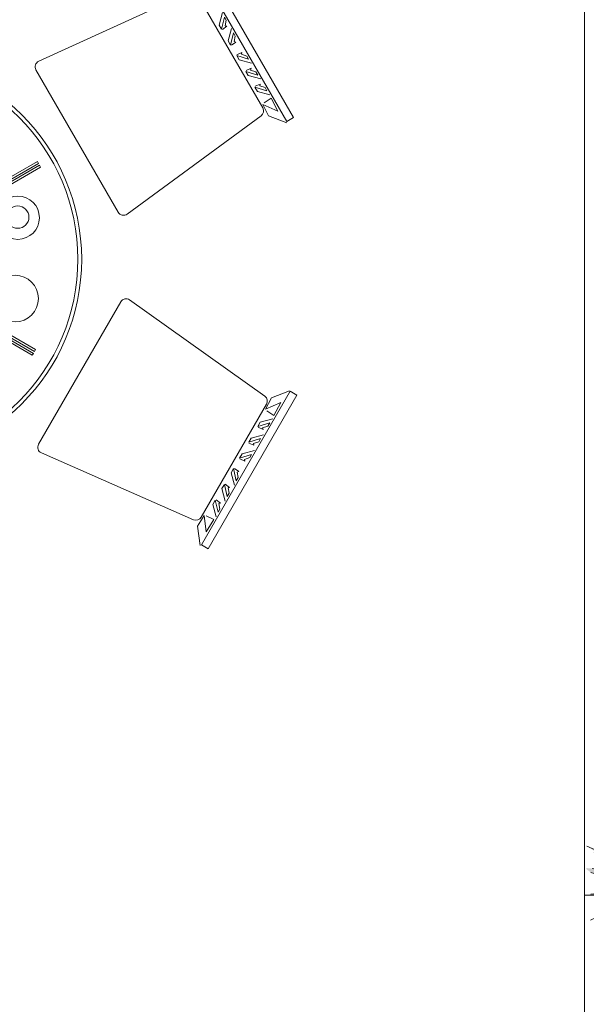
# Model space of a CAD drawing. Units: inches. Extents: x 1239 to 2276906, y 2273 to 321338.
# Tile 4 of 23: x 1482 to 1541, y 2408 to 2510. Entities that reach past the tile are written whole.
import ezdxf

# ---------------------------------------------------------------- set-up
doc = ezdxf.new("R2010")
doc.units = ezdxf.units.IN
for name, color, linetype, lineweight in [('A-ANNO-DIMS', 2, 'Continuous', 18), ('A-FURN', 8, 'Continuous', 13), ('L-PLNT', 94, 'Continuous', 13)]:
    doc.layers.add(name, color=color, linetype=linetype, lineweight=lineweight)
doc.styles.get("Standard").update_dxf_attribs({"font": 'arial.ttf'})
doc.dimstyles.new('ISO-25', dxfattribs={"dimtxt": 4.5, "dimasz": 4, "dimexe": 1.25, "dimexo": 0.625, "dimtad": 1, "dimdec": 1, "dimlunit": 3, "dimtxsty": 'Standard', "dimcen": 2.5, "dimadec": 0, "dimazin": 0, "dimtfac": 1, "dimtdec": 1, "dimtmove": 0, "dimatfit": 3, "dimfxl": 1, "dimarcsym": 0})

# ---------------------------------------------------------------- blocks, each defined once
blk = doc.blocks.new('A$C545C060E')
h = blk.add_hatch(color=256)
h.set_gradient(color1=(31, 127, 0), color2=(45, 179, 0), one_color=1, tint=0.35, name='INVSPHERICAL')
h.paths.add_polyline_path([(0.529, 2.393), (0.645, 2.304), (1.889, 1.967), (0.489, 1.77), (1.843, 1.787), (1.618, 1.643), (0.635, 1.178), (1.063, 1.326), (1.966, 1.643), (1.461, 1.231), (1.869, 1.417), (2.379, 1.664), (2.177, 1.5), (1.446, 1.03), (1.981, 1.358), (1.481, 0.744), (2.376, 1.553), (1.986, 0.848), (2.48, 1.336), (1.85, 0.496), (2.266, 0.842), (2.223, 0.533), (2.243, 0.142), (2.487, 1.093), (2.615, 0.257), (2.655, 1.214), (3.074, 0.284), (3.303, 0), (2.908, 1.003), (2.846, 1.271), (2.929, 1.199), (3.853, 0.038), (3.428, 0.832), (3.973, 0.376), (4.009, 0.393), (3.432, 1.008), (3.923, 0.676), (4.175, 0.507), (4.274, 0.474), (4.155, 0.583), (4.009, 0.757), (3.765, 0.932), (3.662, 1.051), (4.067, 0.828), (4.243, 0.779), (4.238, 0.801), (3.802, 1.133), (4.534, 0.795), (4.591, 0.795), (4.42, 0.899), (4.103, 1.12), (3.786, 1.34), (3.464, 1.533), (3.968, 1.441), (4.415, 1.362), (4.571, 1.335), (4.695, 1.33), (3.997, 1.572), (3.423, 1.771), (4.695, 1.782), (3.833, 1.912), (4.591, 2.011), (3.836, 2.079), (4.706, 2.305), (3.951, 2.263), (4.55, 2.506), (4.555, 2.528), (4.493, 2.517), (3.734, 2.332), (4.197, 2.577), (4.56, 2.833), (3.786, 2.523), (4.363, 2.959), (4.394, 2.997), (4.363, 2.997), (3.558, 2.528), (3.549, 2.536), (4.087, 3.155), (4.254, 3.422), (4.191, 3.389), (3.209, 2.381), (4.046, 3.912), (3.999, 3.874), (3.09, 2.626), (3.547, 3.58), (3.666, 3.934), (3.35, 3.438), (3.017, 2.752), (3.225, 3.411), (3.345, 4.064), (3.243, 3.868), (3.184, 3.754), (2.919, 3.073), (2.986, 3.83), (2.991, 4.097), (2.96, 4.075), (2.742, 2.981), (2.732, 2.92), (2.659, 4.026), (2.633, 4.092), (2.612, 4.005), (2.56, 2.719), (2.3, 4.135), (2.382, 2.743), (2.025, 4.026), (2.02, 3.934), (1.968, 3.917), (2.046, 3.874), (2.185, 2.776), (1.976, 3.197), (1.829, 3.524), (1.673, 3.773), (1.577, 3.963), (1.613, 3.821), (1.751, 3.44), (1.89, 3.059), (2.192, 2.446), (1.345, 3.551), (1.215, 3.683), (1.481, 3.234), (2.006, 2.515), (1.567, 2.769), (0.983, 3.176), (0.731, 3.334), (1.255, 2.901), (1.969, 2.294), (0.912, 2.769), (0.549, 2.927), (1.687, 2.199), (0.675, 2.399), (0.554, 2.409)])
h = blk.add_hatch(color=256)
h.set_gradient(color1=(31, 127, 0), color2=(55, 219, 0), one_color=1, tint=0.43, name='SPHERICAL')
h.paths.add_polyline_path([(3.023, 2.188), (3.114, 2.362), (3.471, 3.049), (3.33, 2.866), (2.618, 1.891), (2.679, 1.855), (2.94, 2.013)])
h = blk.add_hatch(color=256)
h.set_gradient(color1=(31, 127, 0), color2=(45, 179, 0), one_color=1, tint=0.35, name='INVSPHERICAL')
h.paths.add_polyline_path([(0.025, 1.517), (0.098, 1.461), (0.877, 1.25), (0, 1.126), (0.848, 1.137), (0.707, 1.047), (0.092, 0.756), (0.36, 0.848), (0.925, 1.047), (0.609, 0.789), (0.865, 0.905), (1.184, 1.06), (1.058, 0.958), (0.6, 0.663), (0.935, 0.868), (0.622, 0.484), (1.182, 0.99), (0.938, 0.549), (1.247, 0.855), (0.853, 0.328), (1.113, 0.545), (1.086, 0.352), (1.099, 0.106), (1.252, 0.703), (1.332, 0.179), (1.357, 0.779), (1.62, 0.195), (1.763, 0.018), (1.515, 0.646), (1.477, 0.814), (1.529, 0.769), (2.108, 0.042), (1.841, 0.539), (2.183, 0.253), (2.206, 0.264), (1.844, 0.649), (2.152, 0.441), (2.31, 0.335), (2.371, 0.315), (2.297, 0.383), (2.206, 0.492), (2.053, 0.602), (1.988, 0.676), (2.242, 0.537), (2.352, 0.506), (2.349, 0.52), (2.076, 0.728), (2.534, 0.516), (2.57, 0.516), (2.463, 0.581), (2.264, 0.719), (2.066, 0.857), (1.864, 0.978), (2.18, 0.921), (2.46, 0.871), (2.557, 0.854), (2.636, 0.851), (2.198, 1.003), (1.839, 1.127), (2.636, 1.134), (2.095, 1.216), (2.57, 1.277), (2.097, 1.32), (2.642, 1.462), (2.169, 1.435), (2.544, 1.588), (2.548, 1.602), (2.509, 1.595), (2.033, 1.479), (2.323, 1.632), (2.551, 1.793), (2.066, 1.598), (2.427, 1.871), (2.447, 1.895), (2.427, 1.895), (1.923, 1.602), (1.917, 1.606), (2.255, 1.994), (2.359, 2.161), (2.32, 2.141), (1.704, 1.509), (2.229, 2.469), (2.199, 2.445), (1.63, 1.663), (1.916, 2.26), (1.991, 2.482), (1.792, 2.172), (1.584, 1.741), (1.714, 2.155), (1.789, 2.564), (1.726, 2.441), (1.688, 2.369), (1.522, 1.943), (1.565, 2.417), (1.568, 2.584), (1.548, 2.571), (1.412, 1.885), (1.405, 1.847), (1.36, 2.54), (1.343, 2.581), (1.33, 2.526), (1.298, 1.721), (1.135, 2.608), (1.186, 1.736), (0.962, 2.54), (0.959, 2.482), (0.927, 2.472), (0.976, 2.445), (1.063, 1.757), (0.932, 2.02), (0.84, 2.226), (0.742, 2.381), (0.682, 2.501), (0.704, 2.411), (0.791, 2.173), (0.878, 1.934), (1.067, 1.55), (0.537, 2.242), (0.455, 2.325), (0.622, 2.044), (0.951, 1.593), (0.676, 1.752), (0.31, 2.007), (0.152, 2.107), (0.48, 1.835), (0.927, 1.455), (0.265, 1.752), (0.038, 1.851), (0.751, 1.395), (0.117, 1.52), (0.041, 1.527)])
h = blk.add_hatch(color=256)
h.set_gradient(color1=(31, 127, 0), color2=(55, 219, 0), one_color=1, tint=0.43, name='SPHERICAL')
h.paths.add_polyline_path([(1.334, 1.202), (1.372, 1.18), (1.536, 1.279), (1.588, 1.388), (1.645, 1.497), (1.868, 1.928), (1.78, 1.813)])
for p, q in [((2.295, 4.037, -52.769), (2.3, 4.135, -52.769)), ((2.3, 4.135, -52.769), (2.534, 2.893, -52.769)), ((2.612, 4.005, -52.769), (2.633, 4.092, -52.769)), ((2.633, 4.092, -52.769), (2.659, 4.026, -52.769)), ((2.945, 4.01, -52.769), (2.96, 4.075, -52.769)), ((2.96, 4.075, -52.769), (2.991, 4.097, -52.769)), ((2.991, 4.097, -52.769), (2.986, 3.83, -52.769)), ((1.577, 3.963, -52.769), (1.613, 3.821, -52.769)), ((1.673, 3.773, -52.769), (1.577, 3.963, -52.769)), ((1.968, 3.917, -52.769), (2.02, 3.934, -52.769)), ((2.02, 3.934, -52.769), (2.025, 4.026, -52.769)), ((2.025, 4.026, -52.769), (2.389, 2.719, -52.769)), ((2.389, 2.643, -52.769), (2.295, 4.037, -52.769)), ((2.591, 3.329, -52.769), (2.612, 4.005, -52.769)), ((2.659, 4.026, -52.769), (2.732, 2.92, -52.769)), ((2.742, 2.981, -52.769), (2.945, 4.01, -52.769)), ((3.184, 3.754, -52.769), (3.303, 3.983, -52.769)), ((3.345, 4.064, -52.769), (3.225, 3.411, -52.769)), ((3.303, 3.983, -52.769), (3.345, 4.064, -52.769)), ((3.428, 3.553, -52.769), (3.666, 3.934, -52.769)), ((3.666, 3.934, -52.769), (3.547, 3.58, -52.769)), ((1.613, 3.821, -52.769), (1.89, 3.059, -52.769)), ((2.046, 3.874, -52.769), (1.968, 3.917, -52.769)), ((2.103, 3.378, -52.769), (2.046, 3.874, -52.769)), ((2.986, 3.83, -52.769), (2.908, 2.964, -52.769)), ((3.508, 3.479, -52.769), (3.625, 3.884, -52.769)), ((3.558, 3.269, -52.769), (3.999, 3.874, -52.769)), ((4.046, 3.912, -52.769), (3.635, 3.155, -52.769)), ((3.999, 3.874, -52.769), (4.046, 3.912, -52.769)), ((1.215, 3.683, -52.769), (1.481, 3.234, -52.769)), ((1.345, 3.551, -52.769), (1.215, 3.683, -52.769)), ((1.829, 3.524, -52.769), (1.673, 3.773, -52.769)), ((3.095, 3.498, -52.769), (3.184, 3.754, -52.769)), ((1.602, 3.229, -52.769), (1.345, 3.551, -52.769)), ((1.976, 3.197, -52.769), (1.829, 3.524, -52.769)), ((3.198, 3.588, -52.769), (2.75, 2.248, -52.769)), ((2.919, 3.073, -52.769), (3.095, 3.498, -52.769)), ((3.547, 3.58, -52.769), (3.085, 2.626, -52.769)), ((3.35, 3.438, -52.769), (3.428, 3.553, -52.769)), ((2.186, 2.773, -52.769), (2.103, 3.378, -52.769)), ((3.225, 3.411, -52.769), (3.017, 2.752, -52.769)), ((3.298, 3.329, -52.769), (3.35, 3.438, -52.769)), ((3.771, 2.975, -52.769), (4.191, 3.389, -52.769)), ((4.254, 3.422, -52.769), (4.087, 3.155, -52.769)), ((4.191, 3.389, -52.769), (4.254, 3.422, -52.769)), ((0.731, 3.334, -52.769), (1.255, 2.901, -52.769)), ((0.983, 3.176, -52.769), (0.731, 3.334, -52.769)), ((1.481, 3.234, -52.769), (1.819, 2.785, -52.769)), ((2.157, 2.505, -52.769), (1.602, 3.229, -52.769)), ((2.56, 2.719, -52.769), (2.591, 3.329, -52.769)), ((2.849, 3.284, -52.769), (2.65, 1.996, -52.769)), ((3.017, 2.752, -52.769), (3.298, 3.329, -52.769)), ((3.09, 2.626, -52.769), (3.558, 3.269, -52.769)), ((1.567, 2.769, -52.769), (0.983, 3.176, -52.769)), ((1.89, 3.059, -52.769), (2.192, 2.446, -52.769)), ((2.102, 2.927, -52.769), (1.976, 3.197, -52.769)), ((3.635, 3.155, -52.769), (3.209, 2.381, -52.769)), ((4.087, 3.155, -52.769), (3.542, 2.528, -52.769)), ((0.549, 2.927, -52.769), (0.72, 2.785, -52.769)), ((0.912, 2.769, -52.769), (0.549, 2.927, -52.769)), ((2.192, 2.764, -52.769), (2.102, 2.927, -52.769)), ((2.732, 2.92, -52.769), (2.783, 2.212, -52.769)), ((3.471, 3.049, -52.769), (3.114, 2.362, -52.769)), ((3.209, 2.381, -52.769), (3.771, 2.975, -52.769)), ((3.33, 2.866, -52.769), (3.471, 3.049, -52.769)), ((3.558, 2.528, -52.769), (4.327, 2.975, -52.769)), ((4.363, 2.959, -52.769), (3.786, 2.523, -52.769)), ((4.327, 2.975, -52.769), (4.363, 2.997, -52.769)), ((4.394, 2.997, -52.769), (4.363, 2.959, -52.769)), ((4.363, 2.997, -52.769), (4.394, 2.997, -52.769)), ((0.72, 2.785, -52.769), (1.27, 2.43, -52.769)), ((1.522, 2.483, -52.769), (0.912, 2.769, -52.769)), ((1.255, 2.901, -52.769), (1.653, 2.552, -52.769)), ((2.006, 2.515, -52.769), (1.567, 2.769, -52.769)), ((1.819, 2.785, -52.769), (2.016, 2.494, -52.769)), ((2.269, 2.899, -52.769), (2.394, 2.654, -52.769)), ((2.279, 2.724, -52.769), (2.269, 2.899, -52.769)), ((2.534, 2.893, -52.769), (2.56, 2.719, -52.769)), ((2.6, 1.866, -52.769), (3.33, 2.866, -52.769)), ((4.191, 2.692, -52.769), (4.514, 2.822, -52.769)), ((4.56, 2.833, -52.769), (4.197, 2.577, -52.769)), ((4.514, 2.822, -52.769), (4.56, 2.833, -52.769)), ((2.539, 1.864, -52.769), (2.279, 2.724, -52.769)), ((2.394, 2.654, -52.769), (2.55, 2.027, -52.769)), ((3.085, 2.626, -52.769), (2.955, 2.288, -52.769)), ((3.797, 2.528, -52.769), (4.191, 2.692, -52.769)), ((0.682, 2.501), (0.704, 2.411)), ((0.742, 2.381), (0.682, 2.501)), ((0.927, 2.472), (0.959, 2.482)), ((0.959, 2.482), (0.962, 2.54)), ((0.962, 2.54), (1.19, 1.721)), ((1.132, 2.547), (1.135, 2.608)), ((1.19, 1.673), (1.132, 2.547)), ((1.135, 2.608), (1.281, 1.83)), ((1.317, 2.103), (1.33, 2.526)), ((1.33, 2.526), (1.343, 2.581)), ((1.343, 2.581), (1.36, 2.54)), ((1.36, 2.54), (1.405, 1.847)), ((1.412, 1.885), (1.539, 2.53)), ((2.046, 2.261, -52.769), (1.522, 2.483, -52.769)), ((1.539, 2.53), (1.548, 2.571)), ((1.548, 2.571), (1.568, 2.584)), ((1.568, 2.584), (1.565, 2.417)), ((1.653, 2.552, -52.769), (2.087, 2.198, -52.769)), ((1.688, 2.369), (1.763, 2.513)), ((1.789, 2.564), (1.714, 2.155)), ((1.763, 2.513), (1.789, 2.564)), ((1.841, 2.243), (1.991, 2.482)), ((1.991, 2.482), (1.916, 2.26)), ((2.016, 2.494, -52.769), (2.208, 2.129, -52.769)), ((3.786, 2.523, -52.769), (2.674, 1.853, -52.769)), ((3.734, 2.332, -52.769), (4.493, 2.517, -52.769)), ((4.197, 2.577, -52.769), (3.848, 2.381, -52.769)), ((4.55, 2.506, -52.769), (3.854, 2.223, -52.769)), ((4.493, 2.517, -52.769), (4.555, 2.528, -52.769)), ((4.555, 2.528, -52.769), (4.55, 2.506, -52.769)), ((0.554, 2.409, -52.769), (0.529, 2.393, -52.769)), ((0.529, 2.393, -52.769), (0.539, 2.367, -52.769)), ((0.539, 2.367, -52.769), (0.645, 2.304, -52.769)), ((0.675, 2.399, -52.769), (0.554, 2.409, -52.769)), ((1.32, 2.272, -52.769), (0.675, 2.399, -52.769)), ((0.704, 2.411), (0.878, 1.934)), ((0.84, 2.226), (0.742, 2.381)), ((0.976, 2.445), (0.927, 2.472)), ((1.011, 2.134), (0.976, 2.445)), ((1.27, 2.43, -52.769), (1.764, 2.156, -52.769)), ((1.565, 2.417), (1.516, 1.875)), ((1.633, 2.209), (1.688, 2.369)), ((1.891, 2.197), (1.965, 2.451)), ((1.923, 2.066), (2.199, 2.445)), ((2.229, 2.469), (1.971, 1.994)), ((2.199, 2.445), (2.229, 2.469)), ((3.114, 2.362, -52.769), (3.023, 2.188, -52.769)), ((3.848, 2.381, -52.769), (3.734, 2.332, -52.769)), ((0.455, 2.325), (0.622, 2.044)), ((0.537, 2.242), (0.455, 2.325)), ((0.698, 2.04), (0.537, 2.242)), ((0.645, 2.304, -52.769), (1.734, 1.992, -52.769)), ((0.932, 2.02), (0.84, 2.226)), ((1.769, 2.182, -52.769), (1.32, 2.272, -52.769)), ((1.697, 2.266), (1.416, 1.426)), ((1.522, 1.943), (1.633, 2.209)), ((1.916, 2.26), (1.627, 1.663)), ((1.792, 2.172), (1.841, 2.243)), ((2.565, 1.907, -52.769), (2.84, 2.229, -52.769)), ((2.84, 2.229, -52.769), (2.606, 1.885, -52.769)), ((3.878, 2.205, -52.769), (2.857, 1.97, -52.769)), ((3.023, 2.188, -52.769), (2.907, 1.944, -52.769)), ((3.734, 2.25, -52.769), (4.301, 2.283, -52.769)), ((3.949, 2.282, -52.769), (4.001, 2.285, -52.769)), ((4.001, 2.285, -52.769), (4.042, 2.282, -52.769)), ((4.706, 2.305, -52.769), (4.228, 2.169, -52.769)), ((4.301, 2.283, -52.769), (4.706, 2.305, -52.769)), ((0.152, 2.107), (0.48, 1.835)), ((0.31, 2.007), (0.152, 2.107)), ((0.622, 2.044), (0.834, 1.762)), ((1.045, 1.587), (0.698, 2.04)), ((1.063, 1.755), (1.011, 2.134)), ((1.298, 1.721), (1.317, 2.103)), ((1.479, 2.075), (1.354, 1.268)), ((1.714, 2.155), (1.584, 1.741)), ((1.584, 1.741), (1.76, 2.103)), ((1.63, 1.663), (1.923, 2.066)), ((1.76, 2.103), (1.792, 2.172)), ((1.764, 2.156, -52.769), (2.182, 1.902, -52.769)), ((2.009, 2.092, -52.769), (2.476, 1.885, -52.769)), ((2.425, 1.814, -52.769), (2.009, 2.092, -52.769)), ((2.056, 1.881), (2.32, 2.141)), ((2.359, 2.161), (2.255, 1.994)), ((2.32, 2.141), (2.359, 2.161)), ((4.228, 2.169, -52.769), (3.61, 2.027, -52.769)), ((3.807, 2.082, -52.769), (4.264, 2.038, -52.769)), ((3.886, 2.102, -52.769), (3.98, 2.099, -52.769)), ((3.98, 2.099, -52.769), (4.025, 2.091, -52.769)), ((4.264, 2.038, -52.769), (4.534, 2.016, -52.769)), ((0.676, 1.752), (0.31, 2.007)), ((0.878, 1.934), (1.067, 1.55)), ((1.011, 1.851), (0.932, 2.02)), ((1.981, 1.981, -52.769), (1.068, 1.844, -52.769)), ((1.868, 1.928), (1.645, 1.497)), ((1.971, 1.994), (1.704, 1.509)), ((1.734, 1.992, -52.769), (2.006, 1.949, -52.769)), ((1.78, 1.813), (1.868, 1.928)), ((2.255, 1.994), (1.913, 1.602)), ((2.404, 1.881), (2.427, 1.895)), ((2.447, 1.895), (2.427, 1.871)), ((2.427, 1.895), (2.447, 1.895)), ((3.737, 1.239, -52.769), (2.617, 1.892, -52.769)), ((3.516, 1.945, -52.769), (3.028, 2.005, -52.769)), ((4.701, 1.782, -52.769), (3.516, 1.945, -52.769)), ((4.591, 2.011, -52.769), (3.833, 1.912, -52.769)), ((4.534, 2.016, -52.769), (4.591, 2.011, -52.769)), ((0.265, 1.752), (0.038, 1.851)), ((0.145, 1.762), (0.49, 1.54)), ((0.647, 1.573), (0.265, 1.752)), ((0.48, 1.835), (0.729, 1.617)), ((0.64, 1.791, -52.769), (0.489, 1.77, -52.769)), ((0.489, 1.77, -52.769), (1.275, 1.775, -52.769)), ((1.068, 1.844, -52.769), (0.64, 1.791, -52.769)), ((0.951, 1.593), (0.676, 1.752)), ((0.834, 1.762), (0.957, 1.58)), ((1.067, 1.749), (1.011, 1.851)), ((1.115, 1.834), (1.194, 1.68)), ((1.122, 1.724), (1.115, 1.834)), ((1.275, 1.775, -52.769), (2.051, 1.791, -52.769)), ((1.281, 1.83), (1.298, 1.721)), ((1.323, 1.186), (1.78, 1.813)), ((1.405, 1.847), (1.438, 1.404)), ((1.865, 1.801, -52.769), (1.678, 1.675, -52.769)), ((1.704, 1.509), (2.056, 1.881)), ((1.869, 1.417, -52.769), (2.425, 1.814, -52.769)), ((1.87, 1.874, -52.769), (2.276, 1.84, -52.769)), ((1.923, 1.602), (2.404, 1.881)), ((1.966, 1.643, -52.769), (2.107, 1.77, -52.769)), ((2.427, 1.871), (2.066, 1.598)), ((2.32, 1.704), (2.522, 1.786)), ((2.551, 1.793), (2.323, 1.632)), ((2.513, 1.809, -52.769), (2.617, 0.725, -52.769)), ((2.522, 1.786), (2.551, 1.793)), ((2.913, 1.793, -52.769), (2.555, 1.798, -52.769)), ((3.347, 0.787, -52.769), (2.559, 1.822, -52.769)), ((3.504, 1.039, -52.769), (2.584, 1.831, -52.769)), ((3.672, 1.76, -52.769), (2.913, 1.793, -52.769)), ((3.422, 1.766, -52.769), (4.571, 1.379, -52.769)), ((4.695, 1.782, -52.769), (3.672, 1.76, -52.769)), ((0.729, 1.617), (1.001, 1.395)), ((1.285, 1.185), (1.122, 1.724)), ((1.194, 1.68), (1.291, 1.288)), ((1.618, 1.643, -52.769), (1.345, 1.521, -52.769)), ((1.966, 1.643, -52.769), (1.461, 1.231, -52.769)), ((1.627, 1.663), (1.545, 1.451)), ((1.608, 1.516, -52.769), (1.966, 1.643, -52.769)), ((1.678, 1.675, -52.769), (1.618, 1.643, -52.769)), ((2.456, 1.716, -52.769), (1.869, 1.417, -52.769)), ((2.072, 1.602), (2.32, 1.704)), ((2.323, 1.632), (2.105, 1.509)), ((2.177, 1.5, -52.769), (2.379, 1.664, -52.769)), ((2.617, 0.725, -52.769), (2.456, 1.716, -52.769)), ((2.509, 1.595), (2.548, 1.602)), ((2.548, 1.602), (2.544, 1.588)), ((3.443, 1.537, -52.769), (3.178, 1.657, -52.769)), ((0.098, 1.461), (0.78, 1.265)), ((0.521, 1.441), (0.117, 1.52)), ((0.49, 1.54), (0.799, 1.368)), ((0.976, 1.434), (0.647, 1.573)), ((0.957, 1.58), (1.077, 1.352)), ((1.345, 1.521, -52.769), (1.048, 1.379, -52.769)), ((1.063, 1.326, -52.769), (1.608, 1.516, -52.769)), ((2.066, 1.598), (1.369, 1.178)), ((1.446, 1.03, -52.769), (2.177, 1.5, -52.769)), ((1.645, 1.497), (1.588, 1.388)), ((1.986, 0.848, -52.769), (2.376, 1.553, -52.769)), ((2.033, 1.479), (2.509, 1.595)), ((2.105, 1.509), (2.033, 1.479)), ((2.544, 1.588), (2.108, 1.41)), ((2.642, 1.462), (2.343, 1.376)), ((2.388, 1.448), (2.642, 1.462)), ((3.677, 1.493, -52.769), (3.443, 1.537, -52.769)), ((3.448, 1.542, -52.769), (3.786, 1.34, -52.769)), ((4.259, 1.39, -52.769), (3.677, 1.493, -52.769)), ((0.802, 1.385), (0.521, 1.441)), ((1.048, 1.379, -52.769), (0.635, 1.178, -52.769)), ((0.799, 1.368), (1.061, 1.209)), ((0.952, 1.328), (1.245, 1.199)), ((1.213, 1.154), (0.952, 1.328)), ((1.301, 1.212), (1.473, 1.414)), ((1.473, 1.414), (1.327, 1.199)), ((1.981, 1.358, -52.769), (1.481, 0.744, -52.769)), ((2.123, 1.399), (1.484, 1.252)), ((1.588, 1.388), (1.515, 1.235)), ((2.343, 1.376), (1.955, 1.288)), ((2.033, 1.427), (2.388, 1.448)), ((2.079, 1.322), (2.365, 1.294)), ((2.128, 1.335), (2.187, 1.333)), ((2.168, 1.447), (2.2, 1.449)), ((2.187, 1.333), (2.215, 1.328)), ((2.2, 1.449), (2.226, 1.447)), ((2.313, 1.109, -52.769), (2.48, 1.336, -52.769)), ((2.929, 1.199, -52.769), (2.742, 1.362, -52.769)), ((2.819, 1.39, -52.769), (2.908, 1.003, -52.769)), ((3.786, 1.34, -52.769), (4.42, 0.899, -52.769)), ((4.571, 1.335, -52.769), (4.259, 1.39, -52.769)), ((4.571, 1.379, -52.769), (4.695, 1.33, -52.769)), ((4.695, 1.33, -52.769), (4.571, 1.335, -52.769)), ((0.363, 1.173), (0.095, 1.14)), ((0.935, 1.259), (0.363, 1.173)), ((0.78, 1.265), (0.951, 1.239)), ((0.866, 1.192), (1.12, 1.17)), ((1.889, 0.669), (1.312, 1.165)), ((2.035, 0.794), (1.333, 1.203)), ((1.897, 1.236), (1.591, 1.274)), ((2.639, 1.134), (1.897, 1.236)), ((2.57, 1.277), (2.095, 1.216)), ((2.365, 1.294), (2.534, 1.281)), ((2.617, 0.245, -52.769), (2.471, 1.199, -52.769)), ((2.485, 1.067, -52.769), (2.5, 1.22, -52.769)), ((2.534, 1.281), (2.57, 1.277)), ((2.799, 0.97, -52.769), (2.606, 1.297, -52.769)), ((2.658, 1.308, -52.769), (2.617, 0.245, -52.769)), ((3.427, 0.496, -52.769), (2.929, 1.199, -52.769)), ((3.62, 1.074, -52.769), (3.313, 1.248, -52.769)), ((3.802, 1.133, -52.769), (3.479, 1.292, -52.769)), ((0, 1.126), (0.493, 1.13)), ((0.493, 1.13), (0.979, 1.14)), ((0.707, 1.047), (0.537, 0.971)), ((0.925, 1.047), (0.609, 0.789)), ((0.701, 0.967), (0.925, 1.047)), ((0.745, 1.067), (0.707, 1.047)), ((0.862, 1.146), (0.745, 1.067)), ((0.865, 0.905), (1.213, 1.154)), ((1.232, 1.093), (0.865, 0.905)), ((0.925, 1.047), (1.014, 1.126)), ((1.058, 0.958), (1.184, 1.06)), ((1.333, 0.472), (1.232, 1.093)), ((1.268, 1.151), (1.333, 0.472)), ((1.519, 1.141), (1.294, 1.144)), ((1.791, 0.511), (1.297, 1.159)), ((1.994, 1.12), (1.519, 1.141)), ((1.851, 0.98), (1.685, 1.056)), ((1.838, 1.124), (2.557, 0.881)), ((1.85, 0.496, -52.769), (2.313, 1.109, -52.769)), ((2.636, 1.134), (1.994, 1.12)), ((2.308, 1.151, -52.769), (2.223, 0.533, -52.769)), ((2.243, 0.142, -52.769), (2.485, 1.067, -52.769)), ((3.973, 0.376, -52.769), (3.204, 1.019, -52.769)), ((3.324, 1.03, -52.769), (3.599, 0.507, -52.769)), ((4.067, 0.828, -52.769), (3.62, 1.074, -52.769)), ((3.656, 1.057, -52.769), (3.765, 0.932, -52.769)), ((4.243, 0.932, -52.769), (3.802, 1.133, -52.769)), ((3.802, 1.128, -52.769), (4.176, 0.856, -52.769)), ((0.351, 0.881), (0.092, 0.756)), ((0.537, 0.971), (0.351, 0.881)), ((0.36, 0.848), (0.701, 0.967)), ((0.6, 0.663), (1.058, 0.958)), ((0.938, 0.549), (1.182, 0.99)), ((1.46, 0.888), (1.515, 0.646)), ((1.997, 0.953), (1.851, 0.98)), ((1.854, 0.984), (2.066, 0.857)), ((2.362, 0.888), (1.997, 0.953)), ((2.557, 0.854), (2.362, 0.888)), ((2.557, 0.881), (2.636, 0.851)), ((3.074, 0.284, -52.769), (2.799, 0.97, -52.769)), ((2.908, 1.003, -52.769), (3.111, 0.512, -52.769)), ((3.687, 0.839, -52.769), (3.432, 1.008, -52.769)), ((3.432, 1.008, -52.769), (3.786, 0.643, -52.769)), ((3.765, 0.932, -52.769), (4.009, 0.757, -52.769)), ((4.534, 0.795, -52.769), (4.243, 0.932, -52.769)), ((4.42, 0.899, -52.769), (4.591, 0.795, -52.769)), ((0.935, 0.868), (0.622, 0.484)), ((1.14, 0.739), (1.086, 0.352)), ((1.143, 0.713), (1.247, 0.855)), ((1.333, 0.171), (1.242, 0.769)), ((1.251, 0.686), (1.26, 0.782)), ((1.447, 0.625), (1.327, 0.83)), ((1.359, 0.837), (1.333, 0.171)), ((1.529, 0.769), (1.411, 0.871)), ((1.841, 0.328), (1.529, 0.769)), ((1.962, 0.69), (1.77, 0.799)), ((2.076, 0.728), (1.874, 0.827)), ((2.066, 0.857), (2.463, 0.581)), ((2.352, 0.602), (2.076, 0.728)), ((2.636, 0.851), (2.557, 0.854)), ((4.16, 0.512, -52.769), (3.687, 0.839, -52.769)), ((4.009, 0.757, -52.769), (4.155, 0.583, -52.769)), ((4.243, 0.779, -52.769), (4.067, 0.828, -52.769)), ((4.176, 0.856, -52.769), (4.238, 0.801, -52.769)), ((4.238, 0.801, -52.769), (4.243, 0.779, -52.769)), ((4.591, 0.795, -52.769), (4.534, 0.795, -52.769)), ((0.853, 0.328), (1.143, 0.713)), ((1.099, 0.106), (1.251, 0.686)), ((1.62, 0.195), (1.447, 0.625)), ((1.515, 0.646), (1.643, 0.339)), ((2.183, 0.253), (1.701, 0.656)), ((1.776, 0.663), (1.948, 0.335)), ((2.004, 0.543), (1.844, 0.649)), ((1.844, 0.649), (2.066, 0.421)), ((2.242, 0.537), (1.962, 0.69)), ((1.984, 0.68), (2.053, 0.602)), ((2.053, 0.602), (2.206, 0.492)), ((2.076, 0.724), (2.31, 0.554)), ((2.534, 0.516), (2.352, 0.602)), ((3.786, 0.643, -52.769), (4.009, 0.393, -52.769)), ((4.155, 0.583, -52.769), (4.274, 0.474, -52.769)), ((2.3, 0.339), (2.004, 0.543)), ((2.206, 0.492), (2.297, 0.383)), ((2.352, 0.506), (2.242, 0.537)), ((2.31, 0.554), (2.349, 0.52)), ((2.349, 0.52), (2.352, 0.506)), ((2.463, 0.581), (2.57, 0.516)), ((2.57, 0.516), (2.534, 0.516)), ((3.111, 0.512, -52.769), (3.303, 0, -52.769)), ((3.853, 0.038, -52.769), (3.427, 0.496, -52.769)), ((3.599, 0.507, -52.769), (3.786, 0.131, -52.769)), ((4.274, 0.474, -52.769), (4.16, 0.512, -52.769)), ((1.643, 0.339), (1.763, 0.018)), ((2.108, 0.042), (1.841, 0.328)), ((1.948, 0.335), (2.066, 0.1)), ((2.066, 0.421), (2.206, 0.264)), ((2.297, 0.383), (2.371, 0.315)), ((2.371, 0.315), (2.3, 0.339)), ((4.009, 0.393, -52.769), (3.973, 0.376, -52.769)), ((1.763, 0.018), (1.62, 0.195)), ((2.206, 0.264), (2.183, 0.253)), ((3.303, 0, -52.769), (3.074, 0.284, -52.769)), ((2.066, 0.1), (2.108, 0.042)), ((3.786, 0.131, -52.769), (3.853, 0.038, -52.769))]:
    blk.add_line(p, q)
blk = doc.blocks.new('t1')
at = {"xscale": 1200, "yscale": 1200, "zscale": 1200}
blk.add_blockref('A$C545C060E', (1649217, 160231), dxfattribs=at)
blk = doc.blocks.new('A$C45501D90')
for p, q in [((860.5, 776.5), (1093.6, 372.8)), ((1075.7, 362.4), (842.6, 766.1)), ((820.7, 701.7), (424.1, 520.7)), ((1012.8, 397.9), (841.2, 695.1)), ((906.9, 648.4), (898.1, 615.7)), ((904.5, 604.6), (911.9, 636.5)), ((911.9, 636.5), (916.7, 628.2)), ((916.7, 628.2), (914, 613.8)), ((898.1, 615.7), (904.5, 604.6)), ((918.3, 612.6), (906.7, 604)), ((914, 613.8), (918.3, 612.6)), ((930.8, 606.9), (922.1, 574.2)), ((922.1, 574.2), (928.4, 563.1)), ((928.4, 563.1), (935.8, 595.1)), ((942.3, 571.1), (930.6, 562.6)), ((935.8, 595.1), (940.6, 586.8)), ((940.6, 586.8), (937.9, 572.3)), ((937.9, 572.3), (942.3, 571.1)), ((950.8, 524.4), (944.4, 535.5)), ((944.4, 535.5), (975.7, 525.9)), ((958.2, 543.5), (945, 537.7)), ((983.5, 515.7), (950.8, 524.4)), ((957.1, 539.1), (958.2, 543.5)), ((970.9, 534.2), (957.1, 539.1)), ((975.7, 525.9), (970.9, 534.2)), ((416.9, 498.2), (633.1, 123.7)), ((968.4, 494), (999.7, 484.4)), ((974.7, 483), (968.4, 494)), ((982.2, 502), (968.9, 496.2)), ((981, 497.6), (982.2, 502)), ((994.9, 492.7), (981, 497.6)), ((999.7, 484.4), (994.9, 492.7)), ((1007.4, 474.2), (974.7, 483)), ((998.7, 441.5), (992.3, 452.5)), ((992.3, 452.5), (1023.6, 443)), ((1006.1, 460.5), (992.9, 454.7)), ((1031.4, 432.7), (998.7, 441.5)), ((1005, 456.2), (1006.1, 460.5)), ((1018.8, 451.3), (1005, 456.2)), ((1023.6, 443), (1018.8, 451.3)), ((1034.8, 423.6), (1016.3, 411.1)), ((1052.6, 389.6), (1034.8, 423.6)), ((1028.3, 377.5), (1012.9, 407.3)), ((1012.9, 407.3), (1052.6, 389.6)), ((656.3, 118.9), (1008.4, 377.1)), ((1075.9, 358.8), (1028.3, 377.5)), ((1093.6, 372.8), (1075.7, 362.4)), ((255.2, 161.9, 90.8), (420.6, 257.3, 90.8)), ((423.5, 252.2, 90.8), (258.2, 156.7, 90.8)), ((260.9, 152, 90.8), (426.2, 247.5, 90.8)), ((429.2, 242.3, 90.8), (263.8, 146.9, 90.8)), ((420.6, 257.3, 90.8), (423.5, 252.2, 90.8)), ((426.2, 247.5, 90.8), (429.2, 242.3, 90.8)), ((639.9, -111.9), (423.7, -486.4)), ((1018, -360), (663, -106.9)), ((244.9, -151.7, 90.8), (410.3, -247.2, 90.8)), ((413, -242.5, 90.8), (247.6, -147.1, 90.8)), ((250.6, -141.9, 90.8), (415.9, -237.4, 90.8)), ((407.3, -252.4, 90.8), (241.9, -156.9, 90.8)), ((410.3, -247.2, 90.8), (407.3, -252.4, 90.8)), ((415.9, -237.4, 90.8), (413, -242.5, 90.8)), ((851.7, -750.4), (1084.8, -346.6)), ((1102.7, -357), (869.7, -760.7)), ((1083.4, -345.8), (1035.8, -364.4)), ((1084.8, -346.6), (1102.7, -357)), ((851, -678.1), (1022.6, -380.9)), ((1035.8, -364.4), (1020.4, -394.3)), ((1020.4, -394.3), (1060.1, -376.6)), ((1060.1, -376.6), (1042.3, -410.6)), ((1042.3, -410.6), (1023.8, -398.1)), ((1006.2, -428.5), (999.8, -439.5)), ((999.8, -439.5), (1031.1, -430)), ((1038.9, -419.7), (1006.2, -428.5)), ((1026.3, -438.3), (1012.5, -443.1)), ((1031.1, -430), (1026.3, -438.3)), ((1015, -461.2), (982.3, -469.9)), ((1013.6, -447.5), (1000.4, -441.7)), ((1012.5, -443.1), (1013.6, -447.5)), ((982.3, -469.9), (975.9, -481)), ((975.9, -481), (1007.2, -471.4)), ((989.7, -489), (976.5, -483.2)), ((1002.4, -479.7), (988.5, -484.6)), ((988.5, -484.6), (989.7, -489)), ((1007.2, -471.4), (1002.4, -479.7)), ((431.1, -509), (830.8, -684.8)), ((958.3, -511.4), (951.9, -522.5)), ((951.9, -522.5), (983.2, -512.9)), ((991, -502.7), (958.3, -511.4)), ((983.2, -512.9), (978.5, -521.2)), ((965.7, -530.5), (952.5, -524.7)), ((978.5, -521.2), (964.6, -526.1)), ((964.6, -526.1), (965.7, -530.5)), ((929.6, -561.2), (936, -550.1)), ((938.3, -593.9), (929.6, -561.2)), ((936, -550.1), (943.3, -582)), ((949.8, -558.1), (938.1, -549.6)), ((945.4, -559.3), (949.8, -558.1)), ((948.1, -573.8), (945.4, -559.3)), ((905.6, -602.7), (912, -591.6)), ((912, -591.6), (919.4, -623.5)), ((925.8, -599.6), (914.2, -591)), ((943.3, -582), (948.1, -573.8)), ((914.4, -635.4), (905.6, -602.7)), ((919.4, -623.5), (924.2, -615.2)), ((921.5, -600.8), (925.8, -599.6)), ((924.2, -615.2), (921.5, -600.8)), ((881.7, -644.2), (888.1, -633.1)), ((890.4, -676.9), (881.7, -644.2)), ((888.1, -633.1), (895.4, -665)), ((901.9, -641.1), (890.2, -632.5)), ((897.5, -642.2), (901.9, -641.1)), ((900.2, -656.7), (897.5, -642.2)), ((895.4, -665), (900.2, -656.7)), ((841, -701.8), (859.2, -673.6)), ((859.2, -673.6), (863.7, -716.7)), ((863.7, -716.7), (884.3, -684.4)), ((884.3, -684.4), (864.1, -674.6)), ((848.7, -752.3), (841, -701.8)), ((869.7, -760.7), (851.7, -750.4))]:
    blk.add_line(p, q)
for centre, radius in [((0, 0), 537), ((0, 0), 527), ((369, 109.3, 90.8), 56.9), ((368.9, 110.8, 90.8), 29.4), ((361.8, -103.1, 90.8), 61.3)]:
    blk.add_circle(centre, radius)
for centre, start, end in [((430.7, 506.2), 114.5199, 210), ((999, 389.9), 306.2572, 30), ((646.9, 131.7), 210, 306.2572), ((653.7, -119.9), 54.5199, 150), ((1008.8, -373), 330, 54.5199), ((437.5, -494.4), 150, 246.2572), ((837.2, -670.1), 246.2572, 330)]:
    blk.add_arc(centre, 16, start, end)
blk = doc.blocks.new('*D89')
at = {"layer": 'A-ANNO-DIMS', "color": 0, "lineweight": -2, "transparency": 16777216}
for p, q in [((1359.38, 3215.77), (1359.38, 2275.7)), ((1551.38, 3215.77), (1551.38, 2275.7)), ((1363.38, 2276.95), (1547.38, 2276.95))]:
    blk.add_line(p, q, dxfattribs=at)
at = {"layer": 'A-ANNO-DIMS', "color": 0, "transparency": 16777216}
for points in [[(1363.38, 2277.61), (1363.38, 2276.28), (1359.38, 2276.95)], [(1547.38, 2277.61), (1547.38, 2276.28), (1551.38, 2276.95)]]:
    blk.add_solid(points, dxfattribs=at)
at = {"layer": 'Defpoints', "color": 0, "transparency": 16777216}
for p in [(1359.38, 3216.4), (1551.38, 3216.4), (1551.38, 2276.95)]:
    blk.add_point(p, dxfattribs=at)
at = {"layer": 'A-ANNO-DIMS', "color": 0, "transparency": 16777216, "insert": (1455.38, 2279.87), "char_height": 4.5, "attachment_point": 5}
blk.add_mtext('16\'-0"', dxfattribs=at)
blk = doc.blocks.new('*D103')
at = {"layer": 'A-ANNO-DIMS', "color": 0, "lineweight": -2, "transparency": 16777216}
for p, q in [((1539.93, 2607.52), (1247.33, 2607.52)), ((1248.58, 2353.9), (1248.58, 2603.52)), ((1539.93, 2349.9), (1247.33, 2349.9))]:
    blk.add_line(p, q, dxfattribs=at)
at = {"layer": 'A-ANNO-DIMS', "color": 0, "transparency": 16777216}
for points in [[(1247.92, 2603.52), (1249.25, 2603.52), (1248.58, 2607.52)], [(1247.92, 2353.9), (1249.25, 2353.9), (1248.58, 2349.9)]]:
    blk.add_solid(points, dxfattribs=at)
at = {"layer": 'Defpoints', "color": 0, "transparency": 16777216}
for p in [(1248.58, 2607.52), (1540.55, 2607.52), (1540.55, 2349.9)]:
    blk.add_point(p, dxfattribs=at)
at = {"layer": 'A-ANNO-DIMS', "color": 0, "transparency": 16777216, "insert": (1245.63, 2478.71), "char_height": 4.5, "attachment_point": 5, "rotation": 90}
blk.add_mtext('21\'-5 1/2"', dxfattribs=at)

msp = doc.modelspace()

# ---------------------------------------------------------------- linework, layer by layer
at = {"layer": 'L-PLNT'}
msp.add_line((1540.55, 2607.52), (1540.55, 2349.9), dxfattribs=at)

# ---------------------------------------------------------------- block references
at = {"layer": 'A-FURN', "xscale": 0.0393700787401575, "yscale": 0.0393700787401575, "zscale": 0.0393700787401575}
msp.add_blockref('A$C45501D90', (1467.4, 2485.22), dxfattribs=at)
at = {"layer": 'L-PLNT', "xscale": 0.0058381603033249, "yscale": 0.0058381603033249, "zscale": 0.0058381603033249}
msp.add_blockref('t1', (-8087.86, 1476.06, 369.69), dxfattribs=at)

# ---------------------------------------------------------------- dimensions: what is measured, and where the dimension line sits
at = {"layer": 'A-ANNO-DIMS'}
dim = msp.add_linear_dim(base=(1551.38, 2276.95), p1=(1359.38, 3216.4), p2=(1551.38, 3216.4), dimstyle='ISO-25', override={"dimdec": 1, "dimlfac": 1, "dimrnd": 0, "dimzin": 1, "dimdsep": 46, "dimlunit": 4, "dimfrac": 2}, dxfattribs=at)
dim.commit()
dim.dimension.update_dxf_attribs({"geometry": '*D89', "text_midpoint": (1455.38, 2279.87)})
dim = msp.add_linear_dim(base=(1248.58, 2607.52), p1=(1540.55, 2349.9), p2=(1540.55, 2607.52), angle=90, dimstyle='ISO-25', override={"dimdec": 1, "dimlfac": 1, "dimrnd": 0, "dimzin": 1, "dimdsep": 46, "dimlunit": 4, "dimfrac": 2}, dxfattribs=at)
dim.commit()
dim.dimension.update_dxf_attribs({"geometry": '*D103', "text_midpoint": (1245.63, 2478.71)})

doc.saveas('drawing.dxf')
